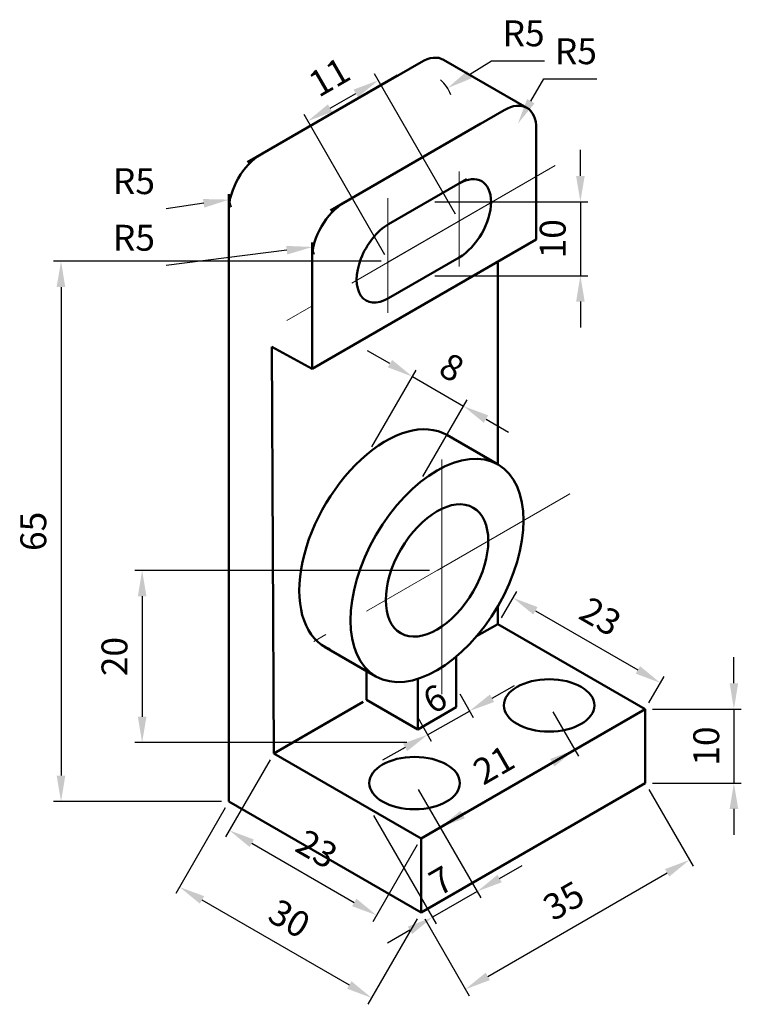
# Model space of a CAD drawing. Units: millimetres. Extents: x 3118 to 3216, y 923 to 1056.
import ezdxf

# ---------------------------------------------------------------- set-up
doc = ezdxf.new("R2010")
doc.units = ezdxf.units.MM
doc.linetypes.add('CENTER', pattern=[50.8, 31.75, -6.35, 6.35, -6.35])
for name, color, linetype, lineweight in [('M-CNTR', 4, 'CENTER', 18), ('M-DIMS', 3, 'Continuous', 25), ('M-OUTL', 7, 'Continuous', 50)]:
    doc.layers.add(name, color=color, linetype=linetype, lineweight=lineweight)
doc.styles.get("Standard").update_dxf_attribs({"font": 'arial.ttf'})
doc.dimstyles.new('AM_ISO$0', dxfattribs={"dimtxt": 3.5, "dimasz": 3.5, "dimexe": 1, "dimexo": 1, "dimgap": 1.5, "dimtad": 1, "dimdsep": 46, "dimtxsty": 'Standard', "dimcen": 0, "dimclrd": 256, "dimclre": 256, "dimclrt": 2, "dimadec": 0, "dimazin": 2, "dimtp": 0.1, "dimtm": 0.1, "dimtfac": 0.71, "dimtdec": 3, "dimtmove": 0, "dimatfit": 3, "dimfxl": 1, "dimlwd": -1, "dimlwe": -1, "dimarcsym": 1})
doc.dimstyles.new('AM_ISO$4', dxfattribs={"dimtxt": 3.5, "dimasz": 3.5, "dimexe": 1, "dimexo": 1, "dimgap": 1.5, "dimtad": 1, "dimtoh": 1, "dimdsep": 46, "dimtxsty": 'Standard', "dimcen": 0, "dimclrd": 256, "dimclre": 256, "dimclrt": 2, "dimadec": 0, "dimazin": 2, "dimtp": 0.1, "dimtm": 0.1, "dimtfac": 0.71, "dimtdec": 3, "dimtofl": 0, "dimtmove": 0, "dimatfit": 0, "dimfxl": 1, "dimlwd": -1, "dimlwe": -1, "dimarcsym": 1})

# ---------------------------------------------------------------- blocks, each defined once
blk = doc.blocks.new('*D3')
at = {"layer": 'Defpoints', "color": 0, "transparency": 16777216}
for p in [(3162.58, 1025.6), (3157.62, 1024.98)]:
    blk.add_point(p, dxfattribs=at)
at = {"layer": 'M-DIMS', "color": 0, "linetype": 'ByBlock', "transparency": 16777216}
blk.add_line((3154.14, 1024.54), (3137.82, 1022.49), dxfattribs=at)
blk.add_arc((3162.58, 1025.6), 5, 180, 198.6126, dxfattribs=at)
at = {"layer": 'M-DIMS', "color": 0, "transparency": 16777216}
blk.add_solid([(3154.07, 1025.12), (3154.21, 1023.96), (3157.62, 1024.98)], dxfattribs=at)
at = {"layer": 'M-DIMS', "color": 0, "transparency": 16777216, "insert": (3133.48, 1025.77), "char_height": 3.5, "attachment_point": 5}
blk.add_mtext('R5', dxfattribs=at)
blk = doc.blocks.new('*D4')
at = {"layer": 'Defpoints', "color": 0, "transparency": 16777216}
for p in [(3151.32, 1032.1), (3146.37, 1031.38)]:
    blk.add_point(p, dxfattribs=at)
at = {"layer": 'M-DIMS', "color": 0, "linetype": 'ByBlock', "transparency": 16777216}
blk.add_line((3142.91, 1030.88), (3137.82, 1030.14), dxfattribs=at)
blk.add_arc((3151.32, 1032.1), 5, 180, 199.7112, dxfattribs=at)
at = {"layer": 'M-DIMS', "color": 0, "transparency": 16777216}
blk.add_solid([(3142.82, 1031.46), (3142.99, 1030.3), (3146.37, 1031.38)], dxfattribs=at)
at = {"layer": 'M-DIMS', "color": 0, "transparency": 16777216, "insert": (3133.48, 1033.42), "char_height": 3.5, "attachment_point": 5}
blk.add_mtext('R5', dxfattribs=at)
blk = doc.blocks.new('*D5')
at = {"layer": 'Defpoints', "color": 0, "transparency": 16777216}
for p in [(3175.88, 1046.45), (3171.63, 1043.83)]:
    blk.add_point(p, dxfattribs=at)
at = {"layer": 'M-DIMS', "color": 0, "linetype": 'ByBlock', "transparency": 16777216}
for p, q in [((3178.86, 1048.29), (3181.84, 1050.13)), ((3181.84, 1050.13), (3189.01, 1050.13))]:
    blk.add_line(p, q, dxfattribs=at)
blk.add_arc((3171.63, 1043.83), 5, 20.2466, 48.5408, dxfattribs=at)
at = {"layer": 'M-DIMS', "color": 0, "transparency": 16777216}
blk.add_solid([(3178.55, 1048.79), (3179.17, 1047.8), (3175.88, 1046.45)], dxfattribs=at)
at = {"layer": 'M-DIMS', "color": 0, "transparency": 16777216, "insert": (3186.17, 1053.41), "char_height": 3.5, "attachment_point": 5}
blk.add_mtext('R5', dxfattribs=at)
blk = doc.blocks.new('*D6')
at = {"layer": 'Defpoints', "color": 0, "transparency": 16777216}
for p in [(3152.38, 956.49), (3172.3, 944.99), (3166.3, 934.6)]:
    blk.add_point(p, dxfattribs=at)
at = {"layer": 'M-DIMS', "color": 0, "linetype": 'ByBlock', "transparency": 16777216}
for p, q in [((3151.88, 955.62), (3145.88, 945.23)), ((3149.41, 944.35), (3163.27, 936.35)), ((3171.8, 944.12), (3165.8, 933.73))]:
    blk.add_line(p, q, dxfattribs=at)
at = {"layer": 'M-DIMS', "color": 0, "transparency": 16777216}
for points in [[(3149.7, 944.85), (3149.12, 943.84), (3146.38, 946.1)], [(3163.56, 936.85), (3162.98, 935.84), (3166.3, 934.6)]]:
    blk.add_solid(points, dxfattribs=at)
at = {"layer": 'M-DIMS', "color": 0, "transparency": 16777216, "insert": (3157.98, 943.19), "char_height": 3.5, "attachment_point": 5, "rotation": 330}
blk.add_mtext('23', dxfattribs=at)
blk = doc.blocks.new('*D7')
at = {"layer": 'Defpoints', "color": 0, "transparency": 16777216}
for p in [(3146.32, 949.99), (3172.3, 934.99), (3165.63, 923.43)]:
    blk.add_point(p, dxfattribs=at)
at = {"layer": 'M-DIMS', "color": 0, "linetype": 'ByBlock', "transparency": 16777216}
for p, q in [((3145.82, 949.12), (3139.15, 937.57)), ((3142.68, 936.68), (3162.6, 925.18)), ((3171.8, 934.12), (3165.13, 922.57))]:
    blk.add_line(p, q, dxfattribs=at)
at = {"layer": 'M-DIMS', "color": 0, "transparency": 16777216}
for points in [[(3142.97, 937.19), (3142.39, 936.18), (3139.65, 938.43)], [(3162.89, 925.69), (3162.31, 924.68), (3165.63, 923.43)]]:
    blk.add_solid(points, dxfattribs=at)
at = {"layer": 'M-DIMS', "color": 0, "transparency": 16777216, "insert": (3154.28, 933.78), "char_height": 3.5, "attachment_point": 5, "rotation": 330}
blk.add_mtext('30', dxfattribs=at)
blk = doc.blocks.new('*D8')
at = {"layer": 'Defpoints', "color": 0, "transparency": 16777216}
for p in [(3202.61, 952.49), (3208.61, 942.1), (3172.3, 934.99)]:
    blk.add_point(p, dxfattribs=at)
at = {"layer": 'M-DIMS', "color": 0, "linetype": 'ByBlock', "transparency": 16777216}
for p, q in [((3203.11, 951.62), (3209.11, 941.23)), ((3181.33, 926.35), (3205.58, 940.35)), ((3172.8, 934.12), (3178.8, 923.73))]:
    blk.add_line(p, q, dxfattribs=at)
at = {"layer": 'M-DIMS', "color": 0, "transparency": 16777216}
for points in [[(3205.29, 940.85), (3205.87, 939.84), (3208.61, 942.1)], [(3181.04, 926.85), (3181.62, 925.84), (3178.3, 924.6)]]:
    blk.add_solid(points, dxfattribs=at)
at = {"layer": 'M-DIMS', "color": 0, "transparency": 16777216, "insert": (3191.81, 936.19), "char_height": 3.5, "attachment_point": 5, "rotation": 30}
blk.add_mtext('35', dxfattribs=at)
blk = doc.blocks.new('*D9')
at = {"layer": 'Defpoints', "color": 0, "transparency": 16777216}
for p in [(3202.61, 962.49), (3202.61, 952.49), (3214.61, 952.49)]:
    blk.add_point(p, dxfattribs=at)
at = {"layer": 'M-DIMS', "color": 0, "linetype": 'ByBlock', "transparency": 16777216}
for p, q in [((3214.61, 965.99), (3214.61, 969.49)), ((3203.61, 962.49), (3215.61, 962.49)), ((3214.61, 962.49), (3214.61, 952.49)), ((3203.61, 952.49), (3215.61, 952.49)), ((3214.61, 948.99), (3214.61, 945.49))]:
    blk.add_line(p, q, dxfattribs=at)
at = {"layer": 'M-DIMS', "color": 0, "transparency": 16777216}
for points in [[(3214.03, 965.99), (3215.19, 965.99), (3214.61, 962.49)], [(3214.03, 948.99), (3215.19, 948.99), (3214.61, 952.49)]]:
    blk.add_solid(points, dxfattribs=at)
at = {"layer": 'M-DIMS', "color": 0, "transparency": 16777216, "insert": (3211.32, 957.49), "char_height": 3.5, "attachment_point": 5, "rotation": 90}
blk.add_mtext('10', dxfattribs=at)
blk = doc.blocks.new('*D10')
at = {"layer": 'Defpoints', "color": 0, "transparency": 16777216}
for p in [(3189.62, 962.99), (3193.08, 956.99), (3171.43, 952.49)]:
    blk.add_point(p, dxfattribs=at)
at = {"layer": 'M-DIMS', "color": 0, "linetype": 'ByBlock', "transparency": 16777216}
for p, q in [((3190.12, 962.12), (3193.58, 956.12)), ((3177.93, 948.24), (3190.05, 955.24)), ((3171.93, 951.62), (3175.4, 945.62))]:
    blk.add_line(p, q, dxfattribs=at)
at = {"layer": 'M-DIMS', "color": 0, "transparency": 16777216}
for points in [[(3189.76, 955.74), (3190.34, 954.73), (3193.08, 956.99)], [(3177.64, 948.74), (3178.22, 947.73), (3174.9, 946.49)]]:
    blk.add_solid(points, dxfattribs=at)
at = {"layer": 'M-DIMS', "color": 0, "transparency": 16777216, "insert": (3182.36, 954.56), "char_height": 3.5, "attachment_point": 5, "rotation": 30}
blk.add_mtext('21', dxfattribs=at)
blk = doc.blocks.new('*D11')
at = {"layer": 'Defpoints', "color": 0, "transparency": 16777216}
for p in [(3171.43, 952.49), (3165.37, 948.99), (3173.83, 934.33)]:
    blk.add_point(p, dxfattribs=at)
at = {"layer": 'M-DIMS', "color": 0, "linetype": 'ByBlock', "transparency": 16777216}
for p, q in [((3171.93, 951.62), (3180.4, 936.96)), ((3165.87, 948.12), (3174.33, 933.46)), ((3182.93, 939.58), (3185.96, 941.33)), ((3179.9, 937.83), (3173.83, 934.33)), ((3170.8, 932.58), (3167.77, 930.83))]:
    blk.add_line(p, q, dxfattribs=at)
at = {"layer": 'M-DIMS', "color": 0, "transparency": 16777216}
for points in [[(3182.64, 940.08), (3183.22, 939.07), (3179.9, 937.83)], [(3170.51, 933.08), (3171.1, 932.07), (3173.83, 934.33)]]:
    blk.add_solid(points, dxfattribs=at)
at = {"layer": 'M-DIMS', "color": 0, "transparency": 16777216, "insert": (3175.24, 938.89), "char_height": 3.5, "attachment_point": 5, "rotation": 30}
blk.add_mtext('7', dxfattribs=at)
blk = doc.blocks.new('*D12')
at = {"layer": 'Defpoints', "color": 0, "transparency": 16777216}
for p in [(3177.06, 965.4), (3171.4, 962.2), (3178.85, 962.23)]:
    blk.add_point(p, dxfattribs=at)
at = {"layer": 'M-DIMS', "color": 0, "linetype": 'ByBlock', "transparency": 16777216}
for p, q in [((3181.9, 963.95), (3184.94, 965.68)), ((3177.55, 964.53), (3179.34, 961.36)), ((3171.89, 961.33), (3173.68, 958.16)), ((3173.19, 959.03), (3178.85, 962.23)), ((3170.14, 957.31), (3167.1, 955.58))]:
    blk.add_line(p, q, dxfattribs=at)
at = {"layer": 'M-DIMS', "color": 0, "transparency": 16777216}
for points in [[(3181.61, 964.46), (3182.19, 963.45), (3178.85, 962.23)], [(3169.86, 957.82), (3170.43, 956.8), (3173.19, 959.03)]]:
    blk.add_solid(points, dxfattribs=at)
at = {"layer": 'M-DIMS', "color": 0, "transparency": 16777216, "insert": (3174.4, 963.49), "char_height": 3.5, "attachment_point": 5, "rotation": 29.4895}
blk.add_mtext('6', dxfattribs=at)
blk = doc.blocks.new('*D13')
at = {"layer": 'Defpoints', "color": 0, "transparency": 16777216}
for p in [(3174.46, 981.24), (3134.59, 957.95), (3171.4, 957.95)]:
    blk.add_point(p, dxfattribs=at)
at = {"layer": 'M-DIMS', "color": 0, "linetype": 'ByBlock', "transparency": 16777216}
for p, q in [((3173.46, 981.24), (3133.59, 981.24)), ((3134.59, 977.74), (3134.59, 961.45)), ((3170.4, 957.95), (3133.59, 957.95))]:
    blk.add_line(p, q, dxfattribs=at)
at = {"layer": 'M-DIMS', "color": 0, "transparency": 16777216}
for points in [[(3134.01, 977.74), (3135.17, 977.74), (3134.59, 981.24)], [(3134.01, 961.45), (3135.17, 961.45), (3134.59, 957.95)]]:
    blk.add_solid(points, dxfattribs=at)
at = {"layer": 'M-DIMS', "color": 0, "transparency": 16777216, "insert": (3131.3, 969.59), "char_height": 3.5, "attachment_point": 5, "rotation": 90}
blk.add_mtext('20', dxfattribs=at)
blk = doc.blocks.new('*D14')
at = {"layer": 'Defpoints', "color": 0, "transparency": 16777216}
for p in [(3166.51, 1047.5), (3177.44, 1028.55), (3167.92, 1023.05)]:
    blk.add_point(p, dxfattribs=at)
at = {"layer": 'M-DIMS', "color": 0, "linetype": 'ByBlock', "transparency": 16777216}
for p, q in [((3176.94, 1029.42), (3166.01, 1048.37)), ((3160.01, 1043.75), (3163.48, 1045.75)), ((3167.42, 1023.92), (3156.48, 1042.87))]:
    blk.add_line(p, q, dxfattribs=at)
at = {"layer": 'M-DIMS', "color": 0, "transparency": 16777216}
for points in [[(3163.18, 1046.26), (3163.77, 1045.24), (3166.51, 1047.5)], [(3159.72, 1044.26), (3160.3, 1043.24), (3156.98, 1042)]]:
    blk.add_solid(points, dxfattribs=at)
at = {"layer": 'M-DIMS', "color": 0, "transparency": 16777216, "insert": (3160.12, 1047.57), "char_height": 3.5, "attachment_point": 5, "rotation": 30}
blk.add_mtext('11', dxfattribs=at)
blk = doc.blocks.new('*D15')
at = {"layer": 'Defpoints', "color": 0, "transparency": 16777216}
for p in [(3173.18, 1031.09), (3173.18, 1021.09), (3193.85, 1021.09)]:
    blk.add_point(p, dxfattribs=at)
at = {"layer": 'M-DIMS', "color": 0, "linetype": 'ByBlock', "transparency": 16777216}
for p, q in [((3193.85, 1034.59), (3193.85, 1038.09)), ((3174.18, 1031.09), (3194.85, 1031.09)), ((3193.85, 1031.09), (3193.85, 1021.09)), ((3174.18, 1021.09), (3194.85, 1021.09)), ((3193.85, 1017.59), (3193.85, 1014.09))]:
    blk.add_line(p, q, dxfattribs=at)
at = {"layer": 'M-DIMS', "color": 0, "transparency": 16777216}
for points in [[(3193.27, 1034.59), (3194.43, 1034.59), (3193.85, 1031.09)], [(3193.27, 1017.59), (3194.43, 1017.59), (3193.85, 1021.09)]]:
    blk.add_solid(points, dxfattribs=at)
at = {"layer": 'M-DIMS', "color": 0, "transparency": 16777216, "insert": (3190.56, 1026.09), "char_height": 3.5, "attachment_point": 5, "rotation": 90}
blk.add_mtext('10', dxfattribs=at)
blk = doc.blocks.new('*D16')
at = {"layer": 'Defpoints', "color": 0, "transparency": 16777216}
for p in [(3178.06, 1003.45), (3165.13, 997.06), (3172.06, 993.06)]:
    blk.add_point(p, dxfattribs=at)
at = {"layer": 'M-DIMS', "color": 0, "linetype": 'ByBlock', "transparency": 16777216}
for p, q in [((3168.1, 1009.2), (3165.07, 1010.95)), ((3165.63, 997.93), (3171.63, 1008.32)), ((3171.13, 1007.45), (3178.06, 1003.45)), ((3172.56, 993.93), (3178.56, 1004.32)), ((3181.09, 1001.7), (3184.12, 999.95))]:
    blk.add_line(p, q, dxfattribs=at)
at = {"layer": 'M-DIMS', "color": 0, "transparency": 16777216}
for points in [[(3168.39, 1009.71), (3167.81, 1008.7), (3171.13, 1007.45)], [(3181.38, 1002.21), (3180.8, 1001.2), (3178.06, 1003.45)]]:
    blk.add_solid(points, dxfattribs=at)
at = {"layer": 'M-DIMS', "color": 0, "transparency": 16777216, "insert": (3176.24, 1008.3), "char_height": 3.5, "attachment_point": 5, "rotation": 330}
blk.add_mtext('8', dxfattribs=at)
blk = doc.blocks.new('*D17')
at = {"layer": 'Defpoints', "color": 0, "transparency": 16777216}
for p in [(3185.39, 1041.65), (3182.89, 1037.33)]:
    blk.add_point(p, dxfattribs=at)
at = {"layer": 'M-DIMS', "color": 0, "linetype": 'ByBlock', "transparency": 16777216}
for p, q in [((3187.15, 1044.68), (3188.9, 1047.71)), ((3188.9, 1047.71), (3196.07, 1047.71))]:
    blk.add_line(p, q, dxfattribs=at)
at = {"layer": 'M-DIMS', "color": 0, "transparency": 16777216}
blk.add_solid([(3186.64, 1044.98), (3187.65, 1044.39), (3185.39, 1041.65)], dxfattribs=at)
at = {"layer": 'M-DIMS', "color": 0, "transparency": 16777216, "insert": (3193.24, 1050.99), "char_height": 3.5, "attachment_point": 5}
blk.add_mtext('R5', dxfattribs=at)
blk = doc.blocks.new('*D18')
at = {"layer": 'Defpoints', "color": 0, "transparency": 16777216}
for p in [(3182.69, 973.99), (3204.66, 966.03), (3202.61, 962.49)]:
    blk.add_point(p, dxfattribs=at)
at = {"layer": 'M-DIMS', "color": 0, "linetype": 'ByBlock', "transparency": 16777216}
for p, q in [((3183.19, 974.85), (3185.24, 978.4)), ((3187.77, 975.78), (3201.63, 967.78)), ((3203.11, 963.35), (3205.16, 966.9))]:
    blk.add_line(p, q, dxfattribs=at)
at = {"layer": 'M-DIMS', "color": 0, "transparency": 16777216}
for points in [[(3188.06, 976.29), (3187.48, 975.28), (3184.74, 977.53)], [(3201.92, 968.29), (3201.33, 967.28), (3204.66, 966.03)]]:
    blk.add_solid(points, dxfattribs=at)
at = {"layer": 'M-DIMS', "color": 0, "transparency": 16777216, "insert": (3196.34, 974.63), "char_height": 3.5, "attachment_point": 5, "rotation": 330}
blk.add_mtext('23', dxfattribs=at)
blk = doc.blocks.new('*D19')
at = {"layer": 'Defpoints', "color": 0, "transparency": 16777216}
for p in [(3167.92, 1023.05), (3123.62, 949.99), (3146.32, 949.99)]:
    blk.add_point(p, dxfattribs=at)
at = {"layer": 'M-DIMS', "color": 0, "linetype": 'ByBlock', "transparency": 16777216}
for p, q in [((3166.92, 1023.05), (3122.62, 1023.05)), ((3123.62, 1019.55), (3123.62, 953.49)), ((3145.32, 949.99), (3122.62, 949.99))]:
    blk.add_line(p, q, dxfattribs=at)
at = {"layer": 'M-DIMS', "color": 0, "transparency": 16777216}
for points in [[(3123.03, 1019.55), (3124.2, 1019.55), (3123.62, 1023.05)], [(3123.03, 953.49), (3124.2, 953.49), (3123.62, 949.99)]]:
    blk.add_solid(points, dxfattribs=at)
at = {"layer": 'M-DIMS', "color": 0, "transparency": 16777216, "insert": (3120.33, 986.52), "char_height": 3.5, "attachment_point": 5, "rotation": 90}
blk.add_mtext('65', dxfattribs=at)

msp = doc.modelspace()

# ---------------------------------------------------------------- linework, layer by layer
at = {"layer": 'M-CNTR'}
for p, q in [((3190.456, 1035.973), (3154.163, 1015.02)), ((3167.811, 1022.9), (3190.456, 1035.973)), ((3177.445, 1022.331), (3177.445, 1035.165)), ((3167.811, 1016.076), (3167.811, 1031.591)), ((3175.116, 996.259), (3175.116, 964.274)), ((3192.419, 991.604), (3157.813, 971.624)), ((3174.464, 981.237), (3192.419, 991.604))]:
    msp.add_line(p, q, dxfattribs=at)
at = {"layer": 'M-OUTL'}
for p, q in [((3172.299, 1049.987), (3150.648, 1037.487)), ((3175.361, 1050.291), (3186.619, 1043.791)), ((3148.818, 1036.431), (3169.129, 1048.157)), ((3183.557, 1043.487), (3161.906, 1030.987)), ((3180.387, 1041.657), (3160.076, 1029.931)), ((3187.887, 1025.987), (3187.887, 1040.987)), ((3187.887, 1025.987), (3187.887, 1037.327)), ((3167.919, 1028.055), (3178.449, 1034.135)), ((3146.318, 1004.987), (3146.318, 1032.101)), ((3157.576, 1008.487), (3187.887, 1025.987)), ((3157.576, 1025.601), (3157.576, 1008.487)), ((3167.919, 1018.055), (3177.445, 1023.555)), ((3182.691, 995.467), (3182.691, 1022.987)), ((3182.691, 995.579), (3182.691, 1022.987)), ((3152.38, 956.487), (3152.123, 1011.487)), ((3152.123, 1011.487), (3157.576, 1008.487)), ((3146.318, 949.987), (3146.318, 1004.987)), ((3175.802, 999.556), (3182.731, 995.556)), ((3182.691, 973.987), (3182.691, 976.396)), ((3182.691, 973.987), (3179.82, 972.33)), ((3202.609, 962.487), (3182.691, 973.987)), ((3166.197, 966.918), (3159.269, 970.918)), ((3177.062, 962.737), (3177.062, 969.575)), ((3164.937, 963.737), (3164.937, 967.645)), ((3171.866, 959.737), (3171.866, 966.575)), ((3152.38, 956.487), (3164.492, 963.48)), ((3164.492, 963.48), (3159.268, 960.464)), ((3171.866, 959.737), (3164.937, 963.737)), ((3171.866, 959.737), (3177.062, 962.737)), ((3172.299, 944.987), (3202.609, 962.487)), ((3202.609, 952.487), (3202.609, 962.487)), ((3159.268, 960.464), (3152.38, 956.487)), ((3152.38, 956.487), (3172.299, 944.987)), ((3172.299, 934.987), (3202.609, 952.487)), ((3172.299, 934.987), (3146.318, 949.987)), ((3172.299, 944.987), (3178.361, 948.487)), ((3172.299, 944.987), (3172.299, 934.987))]:
    msp.add_line(p, q, dxfattribs=at)
for centre, major_axis, start_param, end_param in [((3172.299, 1044.987), (-3.062, -5.303), 3.1415927, 3.9269677), ((3183.557, 1038.487), (-3.062, -5.303), 3.1415927, 3.9269677), ((3183.557, 1038.487), (-3.062, -5.303), 2.3562176, 3.1415927), ((3150.648, 1032.487), (-3.062, -5.303), 3.927014, 5.497764), ((3177.445, 1028.555), (-3.062, -5.303), 7.0685835, 10.2101761), ((3161.906, 1025.987), (-3.062, -5.303), 3.927014, 5.497764), ((3167.919, 1023.055), (-3.062, -5.303), 3.9269908, 7.0685835), ((3167.535, 985.237), (-8.267, -14.319), 3.1415927, 6.3663105)]:
    msp.add_ellipse(centre, major_axis=major_axis, ratio=0.5773503, start_param=start_param, end_param=end_param, dxfattribs=at)
for centre, major_axis in [((3174.464, 981.237), (-8.267, -14.319)), ((3174.464, 981.237), (-4.899, -8.485)), ((3189.619, 962.987), (-6.124, 0)), ((3171.433, 952.487), (-6.124, 0))]:
    msp.add_ellipse(centre, major_axis=major_axis, ratio=0.5773503, dxfattribs=at)

# ---------------------------------------------------------------- dimensions: what is measured, and where the dimension line sits
at = {"layer": 'M-DIMS'}
for center, mpoint, picture, middle in [((3171.629, 1043.827), (3175.882, 1046.455), '*D5', (3186.173, 1050.134)), ((3182.887, 1037.327), (3185.393, 1041.654), '*D17', (3193.235, 1047.712)), ((3151.318, 1032.101), (3146.37, 1031.383), '*D4', (3133.483, 1030.143)), ((3162.576, 1025.601), (3157.615, 1024.978), '*D3', (3133.483, 1022.493))]:
    dim = msp.add_radius_dim(center=center, mpoint=mpoint, dimstyle='AM_ISO$4', override={"dimpost": '', "dimclrd": 0, "dimclre": 0, "dimclrt": 0}, dxfattribs=at)
    dim.commit()
    dim.dimension.update_dxf_attribs({"geometry": picture, "text_midpoint": middle, "dimtype": 164})
for p1, p2, distance, override, picture, middle in [((3167.919, 1023.055), (3177.445, 1028.555), 21.876, {"dimpost": '', "dimclrd": 0, "dimclre": 0, "dimclrt": 0}, '*D14', (3160.115, 1047.571)), ((3173.184, 1031.095), (3173.184, 1021.095), 20.666, {"dimpost": '', "dimclrd": 0, "dimclre": 0, "dimclrt": 0}, '*D15', (3190.563, 1026.095)), ((3165.129, 997.059), (3172.057, 993.059), 12, {"dimpost": '', "dimclrd": 0, "dimclre": 0, "dimclrt": 0}, '*D16', (3176.237, 1008.298)), ((3182.691, 973.987), (3202.609, 962.487), 4.094, {"dimpost": '', "dimclrd": 0, "dimclre": 0, "dimclrt": 0}, '*D18', (3196.341, 974.63)), ((3202.609, 962.487), (3202.609, 952.487), 12, {"dimclrd": 0, "dimclre": 0, "dimclrt": 0}, '*D9', (3211.322, 957.487)), ((3171.433, 952.487), (3189.619, 962.987), -6.928, {"dimclrd": 0, "dimclre": 0, "dimclrt": 0}, '*D10', (3182.361, 954.558)), ((3152.38, 956.487), (3172.299, 944.987), -12, {"dimpost": '', "dimclrd": 0, "dimclre": 0, "dimclrt": 0}, '*D6', (3157.983, 943.193)), ((3171.433, 952.487), (3165.37, 948.987), 16.928, {"dimclrd": 0, "dimclre": 0, "dimclrt": 0}, '*D11', (3175.241, 938.892)), ((3172.299, 934.987), (3202.609, 952.487), -12, {"dimclrd": 0, "dimclre": 0, "dimclrt": 0}, '*D8', (3191.81, 936.193)), ((3146.318, 949.987), (3172.299, 934.987), -13.34, {"dimclrd": 0, "dimclre": 0, "dimclrt": 0}, '*D7', (3154.282, 933.782))]:
    dim = msp.add_aligned_dim(p1=p1, p2=p2, distance=distance, dimstyle='AM_ISO$0', override=override, dxfattribs=at)
    dim.commit()
    dim.dimension.update_dxf_attribs({"geometry": picture, "text_midpoint": middle})
for base, p1, p2, text, picture, middle in [((3123.616, 949.987), (3167.919, 1023.055), (3146.318, 949.987), '65', '*D19', (3120.329, 986.521)), ((3134.591, 957.951), (3174.464, 981.237), (3171.401, 957.951), '20', '*D13', (3131.304, 969.594))]:
    dim = msp.add_linear_dim(base=base, p1=p1, p2=p2, angle=90, text=text, dimstyle='AM_ISO$0', override={"dimpost": '', "dimclrd": 0, "dimclre": 0, "dimclrt": 0}, dxfattribs=at)
    dim.commit()
    dim.dimension.update_dxf_attribs({"geometry": picture, "text_midpoint": middle})
dim = msp.add_aligned_dim(p1=(3171.401, 962.196), p2=(3177.062, 965.397), distance=-3.636, text='6', dimstyle='AM_ISO$0', override={"dimpost": '', "dimclrd": 0, "dimclre": 0, "dimclrt": 0}, dxfattribs=at)
dim.commit()
dim.dimension.update_dxf_attribs({"geometry": '*D12', "text_midpoint": (3174.403, 963.492)})

doc.saveas('drawing.dxf')
